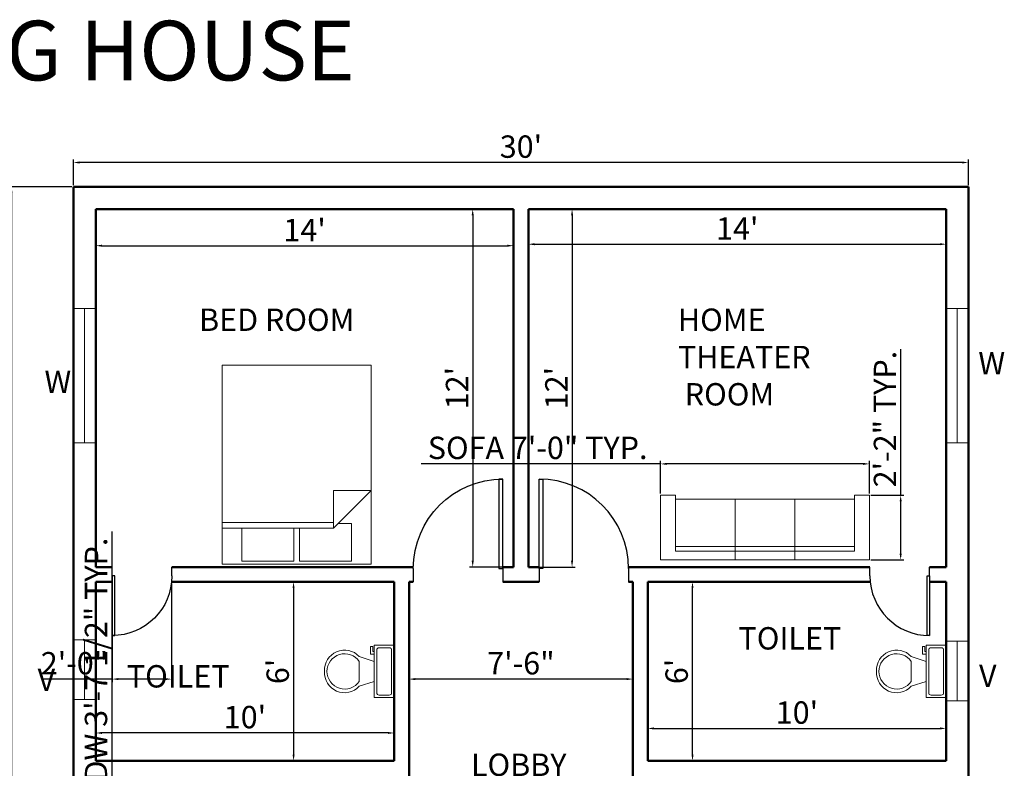
# Model space of a CAD drawing. Units: inches. Extents: x 3587 to 4539, y 1613 to 2440.
# Tile 8 of 8: x 4067 to 4463, y 2139 to 2440. Entities that reach past the tile are written whole.
import ezdxf

# ---------------------------------------------------------------- set-up
doc = ezdxf.new("R2010")
doc.units = ezdxf.units.IN
for name, color, linetype, lineweight in [('A-ANNO-DIMS', 2, 'Continuous', 18), ('A-ANNO-TEXT', 7, 'Continuous', 18), ('A-ANNO-TITL', 7, 'Continuous', 35), ('A-AREA-IDEN', 7, 'Continuous', 25), ('A-DOOR', 3, 'Continuous', 25), ('A-FLOR-FIXT', 9, 'Continuous', 18), ('A-FURN', 8, 'Continuous', 18), ('A-GLAZ', 4, 'Continuous', 20), ('A-WALL', 7, 'Continuous', 50)]:
    doc.layers.add(name, color=color, linetype=linetype, lineweight=lineweight)
doc.styles.get("Standard").update_dxf_attribs({"font": 'arial.ttf'})
doc.dimstyles.new('ISO-25', dxfattribs={"dimtxt": 9, "dimasz": 2.5, "dimexe": 1.25, "dimexo": 0.625, "dimtad": 1, "dimlunit": 3, "dimtxsty": 'Standard', "dimcen": 2.5, "dimadec": 0, "dimazin": 0, "dimtfac": 1, "dimtmove": 0, "dimatfit": 3, "dimfxl": 1, "dimarcsym": 0})

# ---------------------------------------------------------------- blocks, each defined once
blk = doc.blocks.new('*U4')
for p, q in [((0, 0), (0, -6)), ((40, 0), (40, -6))]:
    blk.add_line(p, q)
blk.add_lwpolyline([(0, 0), (0, 40), (1.75, 40), (1.75, 0)], close=True)
blk.add_arc((0, 0), 40, 0, 90)
blk = doc.blocks.new('*U11')
for p, q in [((9.5, -6), (9.5, -2)), ((-10, -8.5), (-8, -8.5)), ((-10, -9.5), (-10, -8.5)), ((-7, -9.5), (-10, -9.5)), ((-8, -8.5), (-8, -8)), ((-7, -8), (-7, -9.5)), ((-4, -8), (-6, -14)), ((4, -8), (6, -14)), ((4, -14), (-4, -14))]:
    blk.add_line(p, q)
blk.add_lwpolyline([(10.5, -8), (10.5, 0), (-10.5, 0), (-10.5, -8)], close=True)
for points in [[(-9.5, -2), (-9.5, -6)], [(8.5, -1), (-8.5, -1)], [(-8.5, -7), (8.5, -7)]]:
    blk.add_lwpolyline(points)
for centre, radius, start, end in [((-8.625, -1.875), 0.8839, 81.8699, 188.1301), ((8.625, -1.875), 0.8839, 351.8699, 98.1301), ((-8.625, -6.125), 0.8839, 171.869898, 278.1301), ((8.625, -6.125), 0.8839, 261.8699, 8.1301), ((-0.4772, -19.9188), 8.0953, 133.01722, 273.38), ((0.0374, -19.8731), 7.127, 124.50543, 269.7), ((-0.0373, -19.8731), 7.127, 270.3, 55.4946), ((0.4773, -19.9188), 8.0953, 266.62, 46.9828)]:
    blk.add_arc(centre, radius, start, end)
blk = doc.blocks.new('Bed - Queen')
for p, q in [((0, -80.00003), (0, 0)), ((0, 0), (59.99999, 0)), ((59.99999, 0), (59.99999, -80.00003)), ((7.99999, -1.2), (28.79998, -1.2)), ((7.99999, -14.4), (7.99999, -1.2)), ((28.79998, -1.2), (28.79998, -14.4)), ((31.19999, -1.2), (51.99999, -1.2)), ((31.19999, -14.4), (31.19999, -1.2)), ((51.99999, -1.2), (51.99999, -16.4)), ((0, -14.4), (44.8, -14.4)), ((59.99999, -29.6), (44.8, -14.4)), ((44.8, -14.4), (44.8, -29.6)), ((44.8, -16.8), (0, -16.8)), ((51.99999, -16.4), (46.79936, -16.4)), ((44.8, -29.6), (59.99999, -29.6)), ((59.99999, -80.00003), (0, -80.00003))]:
    blk.add_line(p, q)
blk = doc.blocks.new('*D40')
at = {"layer": 'A-ANNO-DIMS', "color": 0, "lineweight": -2, "transparency": 16777216}
for p, q in [((4088.12, 2373.56), (4088.12, 2383.96)), ((4448.12, 2373.56), (4448.12, 2383.96)), ((4445.62, 2382.71), (4090.62, 2382.71))]:
    blk.add_line(p, q, dxfattribs=at)
at = {"layer": 'A-ANNO-DIMS', "color": 0, "transparency": 16777216}
for points in [[(4090.62, 2383.12), (4090.62, 2382.29), (4088.12, 2382.71)], [(4445.62, 2383.12), (4445.62, 2382.29), (4448.12, 2382.71)]]:
    blk.add_solid(points, dxfattribs=at)
at = {"layer": 'Defpoints', "color": 0, "transparency": 16777216}
for p in [(4088.12, 2382.71), (4088.12, 2372.93), (4448.12, 2372.93)]:
    blk.add_point(p, dxfattribs=at)
at = {"layer": 'A-ANNO-DIMS', "color": 0, "transparency": 16777216, "insert": (4268.12, 2387.93), "char_height": 9, "attachment_point": 5}
blk.add_mtext("30'", dxfattribs=at)
blk = doc.blocks.new('*D28')
at = {"layer": 'A-ANNO-DIMS', "color": 0, "lineweight": -2, "transparency": 16777216}
for p, q in [((4087.49, 2372.93), (4061.98, 2372.93)), ((4063.23, 2370.43), (4063.23, 1655.43)), ((4087.49, 1652.93), (4061.98, 1652.93))]:
    blk.add_line(p, q, dxfattribs=at)
at = {"layer": 'A-ANNO-DIMS', "color": 0, "transparency": 16777216}
for points in [[(4062.81, 2370.43), (4063.65, 2370.43), (4063.23, 2372.93)], [(4062.81, 1655.43), (4063.65, 1655.43), (4063.23, 1652.93)]]:
    blk.add_solid(points, dxfattribs=at)
at = {"layer": 'Defpoints', "color": 0, "transparency": 16777216}
for p in [(4088.12, 2372.93), (4063.23, 1652.93), (4088.12, 1652.93)]:
    blk.add_point(p, dxfattribs=at)
at = {"layer": 'A-ANNO-DIMS', "color": 0, "transparency": 16777216, "insert": (4058.01, 2019.45), "char_height": 9, "attachment_point": 5, "rotation": 90}
blk.add_mtext("60'", dxfattribs=at)
blk = doc.blocks.new('*D29')
at = {"layer": 'A-ANNO-DIMS', "color": 0, "lineweight": -2, "transparency": 16777216}
for p, q in [((4097.12, 2363.31), (4097.12, 2347.98)), ((4265.12, 2363.31), (4265.12, 2347.98)), ((4099.62, 2349.23), (4262.62, 2349.23))]:
    blk.add_line(p, q, dxfattribs=at)
at = {"layer": 'A-ANNO-DIMS', "color": 0, "transparency": 16777216}
for points in [[(4099.62, 2349.64), (4099.62, 2348.81), (4097.12, 2349.23)], [(4262.62, 2349.64), (4262.62, 2348.81), (4265.12, 2349.23)]]:
    blk.add_solid(points, dxfattribs=at)
at = {"layer": 'Defpoints', "color": 0, "transparency": 16777216}
for p in [(4097.12, 2363.93), (4265.12, 2363.93), (4265.12, 2349.23)]:
    blk.add_point(p, dxfattribs=at)
at = {"layer": 'A-ANNO-DIMS', "color": 0, "transparency": 16777216, "insert": (4181.12, 2354.37), "char_height": 9, "attachment_point": 5}
blk.add_mtext("14'", dxfattribs=at)
blk = doc.blocks.new('*D30')
at = {"layer": 'A-ANNO-DIMS', "color": 0, "lineweight": -2, "transparency": 16777216}
for p, q in [((4264.49, 2363.93), (4247.48, 2363.93)), ((4248.73, 2361.43), (4248.73, 2222.43)), ((4264.49, 2219.93), (4247.48, 2219.93))]:
    blk.add_line(p, q, dxfattribs=at)
at = {"layer": 'A-ANNO-DIMS', "color": 0, "transparency": 16777216}
for points in [[(4248.31, 2361.43), (4249.14, 2361.43), (4248.73, 2363.93)], [(4248.31, 2222.43), (4249.14, 2222.43), (4248.73, 2219.93)]]:
    blk.add_solid(points, dxfattribs=at)
at = {"layer": 'Defpoints', "color": 0, "transparency": 16777216}
for p in [(4265.12, 2363.93), (4248.73, 2219.93), (4265.12, 2219.93)]:
    blk.add_point(p, dxfattribs=at)
at = {"layer": 'A-ANNO-DIMS', "color": 0, "transparency": 16777216, "insert": (4243.58, 2291.93), "char_height": 9, "attachment_point": 5, "rotation": 90}
blk.add_mtext("12'", dxfattribs=at)
blk = doc.blocks.new('*D31')
at = {"layer": 'A-ANNO-DIMS', "color": 0, "lineweight": -2, "transparency": 16777216}
for p, q in [((4271.12, 2363.31), (4271.12, 2348.58)), ((4439.12, 2363.31), (4439.12, 2348.58)), ((4273.62, 2349.83), (4436.62, 2349.83))]:
    blk.add_line(p, q, dxfattribs=at)
at = {"layer": 'A-ANNO-DIMS', "color": 0, "transparency": 16777216}
for points in [[(4273.62, 2350.25), (4273.62, 2349.41), (4271.12, 2349.83)], [(4436.62, 2350.25), (4436.62, 2349.41), (4439.12, 2349.83)]]:
    blk.add_solid(points, dxfattribs=at)
at = {"layer": 'Defpoints', "color": 0, "transparency": 16777216}
for p in [(4271.12, 2363.93), (4439.12, 2363.93), (4439.12, 2349.83)]:
    blk.add_point(p, dxfattribs=at)
at = {"layer": 'A-ANNO-DIMS', "color": 0, "transparency": 16777216, "insert": (4355.12, 2354.97), "char_height": 9, "attachment_point": 5}
blk.add_mtext("14'", dxfattribs=at)
blk = doc.blocks.new('*D32')
at = {"layer": 'A-ANNO-DIMS', "color": 0, "lineweight": -2, "transparency": 16777216}
for p, q in [((4271.74, 2363.93), (4289.94, 2363.93)), ((4288.69, 2361.43), (4288.69, 2222.43)), ((4271.74, 2219.93), (4289.94, 2219.93))]:
    blk.add_line(p, q, dxfattribs=at)
at = {"layer": 'A-ANNO-DIMS', "color": 0, "transparency": 16777216}
for points in [[(4288.27, 2361.43), (4289.1, 2361.43), (4288.69, 2363.93)], [(4288.27, 2222.43), (4289.1, 2222.43), (4288.69, 2219.93)]]:
    blk.add_solid(points, dxfattribs=at)
at = {"layer": 'Defpoints', "color": 0, "transparency": 16777216}
for p in [(4271.12, 2363.93), (4271.12, 2219.93), (4288.69, 2219.93)]:
    blk.add_point(p, dxfattribs=at)
at = {"layer": 'A-ANNO-DIMS', "color": 0, "transparency": 16777216, "insert": (4283.54, 2291.93), "char_height": 9, "attachment_point": 5, "rotation": 90}
blk.add_mtext("12'", dxfattribs=at)
blk = doc.blocks.new('*D33')
at = {"layer": 'A-ANNO-DIMS', "color": 0, "lineweight": -2, "transparency": 16777216}
for p, q in [((4097.12, 2142.56), (4097.12, 2154.41)), ((4217.12, 2142.56), (4217.12, 2154.41)), ((4214.62, 2153.16), (4099.62, 2153.16))]:
    blk.add_line(p, q, dxfattribs=at)
at = {"layer": 'A-ANNO-DIMS', "color": 0, "transparency": 16777216}
for points in [[(4099.62, 2153.58), (4099.62, 2152.75), (4097.12, 2153.16)], [(4214.62, 2153.58), (4214.62, 2152.75), (4217.12, 2153.16)]]:
    blk.add_solid(points, dxfattribs=at)
at = {"layer": 'Defpoints', "color": 0, "transparency": 16777216}
for p in [(4097.12, 2153.16), (4097.12, 2141.93), (4217.12, 2141.93)]:
    blk.add_point(p, dxfattribs=at)
at = {"layer": 'A-ANNO-DIMS', "color": 0, "transparency": 16777216, "insert": (4157.12, 2158.38), "char_height": 9, "attachment_point": 5}
blk.add_mtext("10'", dxfattribs=at)
blk = doc.blocks.new('*D34')
at = {"layer": 'A-ANNO-DIMS', "color": 0, "lineweight": -2, "transparency": 16777216}
for p, q in [((4216.49, 2213.93), (4175.43, 2213.93)), ((4176.68, 2211.43), (4176.68, 2144.43)), ((4216.49, 2141.93), (4175.43, 2141.93))]:
    blk.add_line(p, q, dxfattribs=at)
at = {"layer": 'A-ANNO-DIMS', "color": 0, "transparency": 16777216}
for points in [[(4176.26, 2211.43), (4177.09, 2211.43), (4176.68, 2213.93)], [(4176.26, 2144.43), (4177.09, 2144.43), (4176.68, 2141.93)]]:
    blk.add_solid(points, dxfattribs=at)
at = {"layer": 'Defpoints', "color": 0, "transparency": 16777216}
for p in [(4217.12, 2213.93), (4176.68, 2141.93), (4217.12, 2141.93)]:
    blk.add_point(p, dxfattribs=at)
at = {"layer": 'A-ANNO-DIMS', "color": 0, "transparency": 16777216, "insert": (4171.46, 2177.93), "char_height": 9, "attachment_point": 5, "rotation": 90}
blk.add_mtext("6'", dxfattribs=at)
blk = doc.blocks.new('*D35')
at = {"layer": 'A-ANNO-DIMS', "color": 0, "lineweight": -2, "transparency": 16777216}
for p, q in [((4319.74, 2213.93), (4338.38, 2213.93)), ((4337.13, 2144.43), (4337.13, 2211.43)), ((4319.74, 2141.93), (4338.38, 2141.93))]:
    blk.add_line(p, q, dxfattribs=at)
at = {"layer": 'A-ANNO-DIMS', "color": 0, "transparency": 16777216}
for points in [[(4336.71, 2211.43), (4337.54, 2211.43), (4337.13, 2213.93)], [(4336.71, 2144.43), (4337.54, 2144.43), (4337.13, 2141.93)]]:
    blk.add_solid(points, dxfattribs=at)
at = {"layer": 'Defpoints', "color": 0, "transparency": 16777216}
for p in [(4319.12, 2213.93), (4337.13, 2213.93), (4319.12, 2141.93)]:
    blk.add_point(p, dxfattribs=at)
at = {"layer": 'A-ANNO-DIMS', "color": 0, "transparency": 16777216, "insert": (4331.91, 2177.93), "char_height": 9, "attachment_point": 5, "rotation": 90}
blk.add_mtext("6'", dxfattribs=at)
blk = doc.blocks.new('*D36')
at = {"layer": 'A-ANNO-DIMS', "color": 0, "lineweight": -2, "transparency": 16777216}
for p, q in [((4319.12, 2142.56), (4319.12, 2156.23)), ((4321.62, 2154.98), (4436.62, 2154.98)), ((4439.12, 2142.56), (4439.12, 2156.23))]:
    blk.add_line(p, q, dxfattribs=at)
at = {"layer": 'A-ANNO-DIMS', "color": 0, "transparency": 16777216}
for points in [[(4321.62, 2155.4), (4321.62, 2154.56), (4319.12, 2154.98)], [(4436.62, 2155.4), (4436.62, 2154.56), (4439.12, 2154.98)]]:
    blk.add_solid(points, dxfattribs=at)
at = {"layer": 'Defpoints', "color": 0, "transparency": 16777216}
for p in [(4439.12, 2154.98), (4319.12, 2141.93), (4439.12, 2141.93)]:
    blk.add_point(p, dxfattribs=at)
at = {"layer": 'A-ANNO-DIMS', "color": 0, "transparency": 16777216, "insert": (4379.12, 2160.2), "char_height": 9, "attachment_point": 5}
blk.add_mtext("10'", dxfattribs=at)
blk = doc.blocks.new('SOFA-3-SEAT-84IN')
for p, q in [((0, 0), (0, 84)), ((26, 78), (3.47, 78)), ((3.47, 78), (3.47, 6)), ((5.38, 6), (5.38, 78)), ((24.44, 6), (24.44, 78)), ((24.44, 54), (0, 54)), ((24.44, 30), (0, 30)), ((26, 6), (3.47, 6))]:
    blk.add_line(p, q)
for points in [[(0, 84), (26, 84), (26, 78)], [(26, 6), (26, 0), (0, 0)]]:
    blk.add_lwpolyline(points)
blk = doc.blocks.new('WINDOW-54IN')
for p, q in [((9, 54), (0, 54)), ((4.5, 54), (4.5, 0)), ((9, 0), (0, 0))]:
    blk.add_line(p, q)
blk = doc.blocks.new('VENT-24IN')
for p, q in [((9, 24), (0, 24)), ((4.5, 0), (4.5, 24)), ((9, 0), (0, 0))]:
    blk.add_line(p, q)
blk = doc.blocks.new('*D58')
at = {"layer": 'A-ANNO-DIMS', "color": 0, "lineweight": -2, "transparency": 16777216}
for p, q in [((4103.66, 2117.93), (4103.66, 2234.19)), ((4097.74, 2117.93), (4104.91, 2117.93)), ((4103.66, 2076.82), (4103.66, 2115.43)), ((4097.74, 2074.32), (4104.91, 2074.32))]:
    blk.add_line(p, q, dxfattribs=at)
at = {"layer": 'A-ANNO-DIMS', "color": 0, "transparency": 16777216}
for points in [[(4103.24, 2115.43), (4104.07, 2115.43), (4103.66, 2117.93)], [(4103.24, 2076.82), (4104.07, 2076.82), (4103.66, 2074.32)]]:
    blk.add_solid(points, dxfattribs=at)
at = {"layer": 'Defpoints', "color": 0, "transparency": 16777216}
for p in [(4097.12, 2117.93), (4103.66, 2117.93), (4097.12, 2074.32)]:
    blk.add_point(p, dxfattribs=at)
at = {"layer": 'A-ANNO-DIMS', "color": 0, "transparency": 16777216, "insert": (4098.38, 2177.31), "char_height": 9, "attachment_point": 5, "rotation": 90}
blk.add_mtext('WDW 3\'-7 1/2" TYP.', dxfattribs=at)
blk = doc.blocks.new('*D64')
at = {"layer": 'A-ANNO-DIMS', "color": 0, "lineweight": -2, "transparency": 16777216}
for p, q in [((4324.24, 2261.43), (4227.95, 2261.43)), ((4324.24, 2249.45), (4324.24, 2262.68)), ((4405.74, 2261.43), (4326.74, 2261.43)), ((4408.24, 2249.45), (4408.24, 2262.68))]:
    blk.add_line(p, q, dxfattribs=at)
at = {"layer": 'A-ANNO-DIMS', "color": 0, "transparency": 16777216}
for points in [[(4326.74, 2261.84), (4326.74, 2261.01), (4324.24, 2261.43)], [(4405.74, 2261.84), (4405.74, 2261.01), (4408.24, 2261.43)]]:
    blk.add_solid(points, dxfattribs=at)
at = {"layer": 'Defpoints', "color": 0, "transparency": 16777216}
for p in [(4324.24, 2261.43), (4324.24, 2248.83), (4408.24, 2248.83)]:
    blk.add_point(p, dxfattribs=at)
at = {"layer": 'A-ANNO-DIMS', "color": 0, "transparency": 16777216, "insert": (4274.84, 2266.71), "char_height": 9, "attachment_point": 5}
blk.add_mtext('SOFA 7\'-0" TYP.', dxfattribs=at)
blk = doc.blocks.new('*D65')
at = {"layer": 'A-ANNO-DIMS', "color": 0, "lineweight": -2, "transparency": 16777216}
for p, q in [((4420.84, 2248.83), (4420.84, 2307.59)), ((4408.87, 2248.83), (4422.09, 2248.83)), ((4420.84, 2225.33), (4420.84, 2246.33)), ((4408.87, 2222.83), (4422.09, 2222.83))]:
    blk.add_line(p, q, dxfattribs=at)
at = {"layer": 'A-ANNO-DIMS', "color": 0, "transparency": 16777216}
for points in [[(4420.42, 2246.33), (4421.26, 2246.33), (4420.84, 2248.83)], [(4420.42, 2225.33), (4421.26, 2225.33), (4420.84, 2222.83)]]:
    blk.add_solid(points, dxfattribs=at)
at = {"layer": 'Defpoints', "color": 0, "transparency": 16777216}
for p in [(4408.24, 2248.83), (4420.84, 2248.83), (4408.24, 2222.83)]:
    blk.add_point(p, dxfattribs=at)
at = {"layer": 'A-ANNO-DIMS', "color": 0, "transparency": 16777216, "insert": (4415.69, 2279.46), "char_height": 9, "attachment_point": 5, "rotation": 90}
blk.add_mtext('2\'-2" TYP.', dxfattribs=at)
blk = doc.blocks.new('*D90')
at = {"layer": 'A-ANNO-DIMS', "color": 0, "lineweight": -2, "transparency": 16777216}
for p, q in [((4103.73, 2213.31), (4103.73, 2173.58)), ((4127.61, 2213.31), (4127.61, 2173.58)), ((4103.73, 2174.83), (4075.9, 2174.83)), ((4125.11, 2174.83), (4106.23, 2174.83))]:
    blk.add_line(p, q, dxfattribs=at)
at = {"layer": 'A-ANNO-DIMS', "color": 0, "transparency": 16777216}
for points in [[(4106.23, 2175.25), (4106.23, 2174.42), (4103.73, 2174.83)], [(4125.11, 2175.25), (4125.11, 2174.42), (4127.61, 2174.83)]]:
    blk.add_solid(points, dxfattribs=at)
at = {"layer": 'Defpoints', "color": 0, "transparency": 16777216}
for p in [(4103.73, 2213.93), (4127.61, 2213.93), (4103.73, 2174.83)]:
    blk.add_point(p, dxfattribs=at)
at = {"layer": 'A-ANNO-DIMS', "color": 0, "transparency": 16777216, "insert": (4088.57, 2180.05), "char_height": 9, "attachment_point": 5}
blk.add_mtext('2\'-0"', dxfattribs=at)
blk = doc.blocks.new('*D95')
at = {"layer": 'A-ANNO-DIMS', "color": 0, "lineweight": -2, "transparency": 16777216}
for p, q in [((4223.12, 2213.31), (4223.12, 2173.58)), ((4313.12, 2213.31), (4313.12, 2173.58)), ((4310.62, 2174.83), (4225.62, 2174.83))]:
    blk.add_line(p, q, dxfattribs=at)
at = {"layer": 'A-ANNO-DIMS', "color": 0, "transparency": 16777216}
for points in [[(4225.62, 2175.25), (4225.62, 2174.42), (4223.12, 2174.83)], [(4310.62, 2175.25), (4310.62, 2174.42), (4313.12, 2174.83)]]:
    blk.add_solid(points, dxfattribs=at)
at = {"layer": 'Defpoints', "color": 0, "transparency": 16777216}
for p in [(4223.12, 2213.93), (4313.12, 2213.93), (4223.12, 2174.83)]:
    blk.add_point(p, dxfattribs=at)
at = {"layer": 'A-ANNO-DIMS', "color": 0, "transparency": 16777216, "insert": (4268.12, 2180.05), "char_height": 9, "attachment_point": 5}
blk.add_mtext('7\'-6"', dxfattribs=at)

msp = doc.modelspace()

# ---------------------------------------------------------------- linework, layer by layer
at = {"layer": 'A-WALL'}
for p, q in [((4448.116, 2372.933), (4088.116, 2372.933)), ((4088.116, 2372.933), (4088.116, 1652.933)), ((4448.116, 2372.933), (4448.116, 1652.933)), ((4265.116, 2363.933), (4097.116, 2363.933)), ((4097.116, 2363.933), (4097.116, 2219.933)), ((4265.116, 2363.933), (4265.116, 2219.933)), ((4439.116, 2363.933), (4271.116, 2363.933)), ((4271.116, 2363.933), (4271.116, 2219.933)), ((4439.116, 2363.933), (4439.116, 2219.933)), ((4103.732, 2219.933), (4097.116, 2219.933)), ((4224.84, 2219.933), (4127.732, 2219.933)), ((4265.116, 2219.933), (4260.835, 2219.933)), ((4275.396, 2219.933), (4271.116, 2219.933)), ((4408.499, 2219.933), (4311.391, 2219.933)), ((4439.116, 2219.933), (4432.499, 2219.933)), ((4103.732, 2213.933), (4097.116, 2213.933)), ((4097.116, 2213.933), (4097.116, 2141.933)), ((4217.116, 2213.933), (4127.612, 2213.933)), ((4217.116, 2213.933), (4217.116, 2141.933)), ((4224.835, 2213.933), (4223.116, 2213.933)), ((4223.116, 2213.933), (4223.116, 2135.933)), ((4265.116, 2213.933), (4260.835, 2213.933)), ((4275.396, 2213.933), (4265.116, 2213.933)), ((4313.116, 2213.933), (4311.396, 2213.933)), ((4313.116, 2213.933), (4313.116, 2135.933)), ((4408.619, 2213.933), (4319.116, 2213.933)), ((4319.116, 2213.933), (4319.116, 2141.933)), ((4439.116, 2213.933), (4432.499, 2213.933)), ((4439.116, 2213.933), (4439.116, 2141.933)), ((4217.116, 2141.933), (4097.116, 2141.933)), ((4439.116, 2141.933), (4319.116, 2141.933))]:
    msp.add_line(p, q, dxfattribs=at)

# ---------------------------------------------------------------- block references
at = {"layer": 'A-DOOR', "yscale": 0.9, "zscale": 0.9}
for p, xscale in [((4260.835, 2219.333), -0.9), ((4275.396, 2219.333), 0.9)]:
    msp.add_blockref('*U4', p, dxfattribs=dict(at, xscale=xscale))
at = {"layer": 'A-DOOR', "yscale": 0.6, "zscale": 0.6, "rotation": 180}
for p, xscale in [((4103.732, 2216.333), -0.6), ((4432.499, 2216.333), 0.6)]:
    msp.add_blockref('*U4', p, dxfattribs=dict(at, xscale=xscale))
at = {"layer": 'A-FLOR-FIXT', "rotation": 270}
for p in [(4217.116, 2177.933), (4439.116, 2177.933)]:
    msp.add_blockref('*U11', p, dxfattribs=at)
at = {"layer": 'A-FURN', "xscale": -1, "rotation": 180}
msp.add_blockref('Bed - Queen', (4147.916, 2221.11), dxfattribs=at)
at = {"layer": 'A-FURN', "rotation": 90.00000000000003}
msp.add_blockref('SOFA-3-SEAT-84IN', (4408.241, 2222.826), dxfattribs=at)
at = {"layer": 'A-GLAZ'}
for name, p in [('WINDOW-54IN', (4088.115, 2269.932)), ('WINDOW-54IN', (4439.115, 2269.932)), ('VENT-24IN', (4088.115, 2166.578)), ('VENT-24IN', (4439.115, 2166.139))]:
    msp.add_blockref(name, p, dxfattribs=at)

# ---------------------------------------------------------------- texts
at = {"layer": 'A-ANNO-TEXT', "char_height": 9, "attachment_point": 1}
for s, width, insert in [('W', 47.85632, (4452.073, 2306.421)), ('W', 47.85632, (4076.488, 2299.001)), ('V', 55.41427, (4073.724, 2179.076)), ('V', 55.41427, (4452.344, 2180.666))]:
    msp.add_mtext_dynamic_manual_height_columns(s, width=width, gutter_width=12.5, heights=[0], dxfattribs=dict(at, insert=insert))
at = {"layer": 'A-ANNO-TITL', "insert": (3883.118, 2439.751), "char_height": 24, "attachment_point": 1}
msp.add_mtext_dynamic_manual_height_columns('EAST FACING HOUSE', width=425.00601, gutter_width=12.5, heights=[0], dxfattribs=at)
at = {"layer": 'A-AREA-IDEN', "char_height": 9, "attachment_point": 1}
for s, width, insert in [('BED ROOM', 136.86909, (4138.673, 2323.938)), ('HOME\\PTHEATER\\P ROOM', 136.86909, (4331.246, 2323.938)), ('TOILET', 135.91196, (4355.612, 2195.74)), ('TOILET', 135.91196, (4109.621, 2180.453)), ('LOBBY', 107.19817, (4248.017, 2144.864))]:
    msp.add_mtext_dynamic_manual_height_columns(s, width=width, gutter_width=12.5, heights=[0], dxfattribs=dict(at, insert=insert))

# ---------------------------------------------------------------- dimensions: what is measured, and where the dimension line sits
at = {"layer": 'A-ANNO-DIMS'}
for base, p1, p2, picture, middle in [((4088.116, 2382.707), (4448.116, 2372.933), (4088.116, 2372.933), '*D40', (4268.116, 2387.93)), ((4265.116, 2349.226), (4097.116, 2363.933), (4265.116, 2363.933), '*D29', (4181.116, 2354.37)), ((4439.116, 2349.831), (4271.116, 2363.933), (4439.116, 2363.933), '*D31', (4355.116, 2354.975)), ((4439.116, 2154.979), (4319.116, 2141.933), (4439.116, 2141.933), '*D36', (4379.116, 2160.2)), ((4097.116, 2153.164), (4217.116, 2141.933), (4097.116, 2141.933), '*D33', (4157.116, 2158.384))]:
    dim = msp.add_linear_dim(base=base, p1=p1, p2=p2, dimstyle='ISO-25', override={"dimclrd": 0, "dimclre": 0, "dimclrt": 0}, dxfattribs=at)
    dim.commit()
    dim.dimension.update_dxf_attribs({"geometry": picture, "text_midpoint": middle})
dim = msp.add_linear_dim(base=(4063.23, 1652.933), p1=(4088.116, 2372.933), p2=(4088.116, 1652.933), angle=90, dimstyle='ISO-25', override={"dimclrd": 0, "dimclre": 0, "dimclrt": 0}, dxfattribs=at)
dim.commit()
dim.dimension.update_dxf_attribs({"geometry": '*D28', "text_midpoint": (4063.23, 2019.453), "dimtype": 160})
for base, p1, p2, angle, override, picture, middle in [((4248.727, 2219.933), (4265.116, 2363.933), (4265.116, 2219.933), 90, {"dimclrd": 0, "dimclre": 0, "dimclrt": 0}, '*D30', (4243.584, 2291.933)), ((4288.688, 2219.933), (4271.116, 2363.933), (4271.116, 2219.933), 90, {"dimclrd": 0, "dimclre": 0, "dimclrt": 0}, '*D32', (4283.545, 2291.933)), ((4103.732, 2174.833), (4127.612, 2213.933), (4103.732, 2213.933), 180, {"dimdec": 1, "dimlfac": 1, "dimrnd": 0, "dimzin": 1, "dimdsep": 46, "dimlunit": 4, "dimfrac": 2}, '*D90', (4088.568, 2180.053)), ((4176.677, 2141.933), (4217.116, 2213.933), (4217.116, 2141.933), 90, {"dimclrd": 0, "dimclre": 0, "dimclrt": 0}, '*D34', (4171.457, 2177.933)), ((4223.116, 2174.833), (4313.116, 2213.933), (4223.116, 2213.933), 180, {"dimdec": 1, "dimlfac": 1, "dimrnd": 0, "dimzin": 1, "dimdsep": 46, "dimlunit": 4, "dimfrac": 2}, '*D95', (4268.116, 2180.053)), ((4337.125, 2213.933), (4319.116, 2141.933), (4319.116, 2213.933), 90, {"dimclrd": 0, "dimclre": 0, "dimclrt": 0}, '*D35', (4331.905, 2177.933))]:
    dim = msp.add_linear_dim(base=base, p1=p1, p2=p2, angle=angle, dimstyle='ISO-25', override=override, dxfattribs=at)
    dim.commit()
    dim.dimension.update_dxf_attribs({"geometry": picture, "text_midpoint": middle})
for base, p1, p2, angle, text, picture, middle in [((4420.84, 2248.826), (4408.24, 2222.826), (4408.24, 2248.826), 90, '<> TYP.', '*D65', (4415.694, 2279.457)), ((4324.24, 2261.426), (4408.24, 2248.826), (4324.24, 2248.826), 180, 'SOFA <> TYP.', '*D64', (4274.844, 2266.707)), ((4103.657, 2117.933), (4097.116, 2074.325), (4097.116, 2117.933), 90, 'WDW <> TYP.', '*D58', (4098.375, 2177.311))]:
    dim = msp.add_linear_dim(base=base, p1=p1, p2=p2, angle=angle, text=text, dimstyle='ISO-25', override={"dimdec": 1, "dimlfac": 1, "dimrnd": 0, "dimzin": 1, "dimdsep": 46, "dimlunit": 4, "dimfrac": 2}, dxfattribs=at)
    dim.commit()
    dim.dimension.update_dxf_attribs({"geometry": picture, "text_midpoint": middle})

doc.saveas('drawing.dxf')
